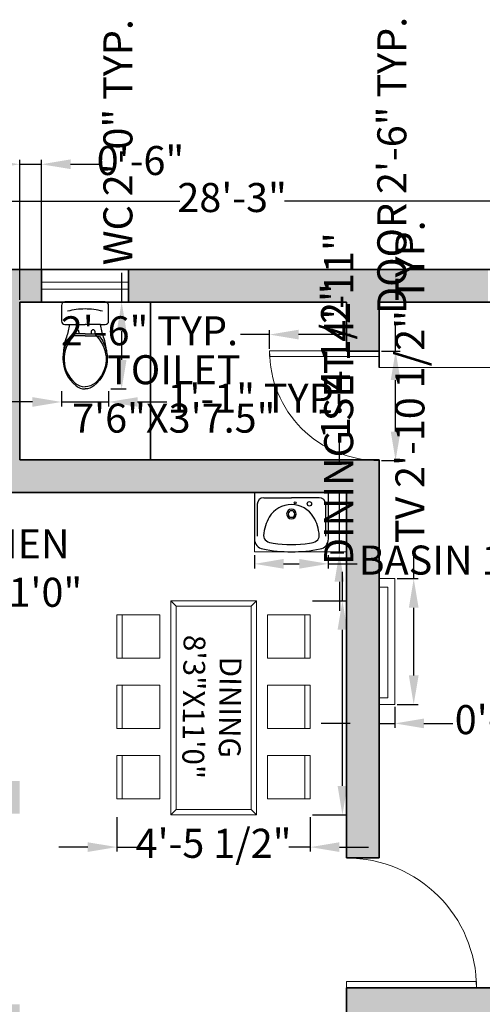
# Model space of a CAD drawing. Units: inches. Extents: x 2408 to 5087, y 2429 to 5085.
# Tile 11 of 12: x 2595 to 2723, y 2815 to 3086. Entities that reach past the tile are written whole.
import ezdxf

# ---------------------------------------------------------------- set-up
doc = ezdxf.new("R2010")
doc.units = ezdxf.units.IN
for name, color, linetype, lineweight in [('A-ANNO-DIMS', 2, 'Continuous', 18), ('A-AREA-IDEN', 6, 'Continuous', 18), ('A-DOOR', 3, 'Continuous', 18), ('A-EQPM', 53, 'Continuous', 18), ('A-FLOR-CASE', 8, 'Continuous', 18), ('A-FLOR-FIXT', 9, 'Continuous', 18), ('A-FURN', 72, 'Continuous', 18), ('A-GLAZ', 4, 'Continuous', 18), ('A-WALL', 7, 'Continuous', 35), ('A-WALL-PATT', 252, 'Continuous', 13)]:
    doc.layers.add(name, color=color, linetype=linetype, lineweight=lineweight)
for name, color, linetype in [('Washbasin-detail', 251, 'Continuous'), ('Washbasin-outline', 250, 'Continuous'), ('WC-Detail_dwgmodels.com', 251, 'Continuous'), ('WC-Outline_dwgmodels.com', 250, 'Continuous')]:
    doc.layers.add(name, color=color, linetype=linetype)
doc.styles.get("Standard").update_dxf_attribs({"font": 'arial.ttf'})
doc.dimstyles.new('ISO-25', dxfattribs={"dimtxt": 8, "dimasz": 8, "dimexe": 1.25, "dimexo": 0.625, "dimtad": 0, "dimdec": 1, "dimlunit": 4, "dimtxsty": 'Standard', "dimcen": 2.5, "dimadec": 0, "dimazin": 0, "dimtfac": 1, "dimtdec": 1, "dimtmove": 0, "dimatfit": 3, "dimfxl": 1, "dimarcsym": 0})

# ---------------------------------------------------------------- blocks, each defined once
blk = doc.blocks.new('*D1')
at = {"layer": 'A-ANNO-DIMS', "color": 0, "lineweight": -2, "transparency": 16777216}
for p, q in [((2484.49, 3017.68), (2484.49, 3037.05)), ((2492.49, 3035.8), (2639.56, 3035.8)), ((2815.49, 3035.8), (2668.43, 3035.8)), ((2823.49, 3017.68), (2823.49, 3037.05))]:
    blk.add_line(p, q, dxfattribs=at)
at = {"layer": 'A-ANNO-DIMS', "color": 0, "transparency": 16777216}
for points in [[(2492.49, 3037.13), (2492.49, 3034.47), (2484.49, 3035.8)], [(2815.49, 3037.13), (2815.49, 3034.47), (2823.49, 3035.8)]]:
    blk.add_solid(points, dxfattribs=at)
at = {"layer": 'Defpoints', "color": 0, "transparency": 16777216}
for p in [(2823.49, 3035.8), (2484.49, 3017.05), (2823.49, 3017.05)]:
    blk.add_point(p, dxfattribs=at)
at = {"layer": 'A-ANNO-DIMS', "color": 0, "transparency": 16777216, "insert": (2653.99, 3035.8), "char_height": 8, "attachment_point": 5}
blk.add_mtext('28\'-3"', dxfattribs=at)
blk = doc.blocks.new('dt')
for p, q in [((2249.04, 2869.72), (2247.08, 2871.69)), ((2278.57, 2871.69), (2276.6, 2869.72)), ((2229.22, 2850.55), (2229.22, 2866.48)), ((2296.41, 2850.55), (2296.41, 2866.48)), ((2229.22, 2824.7), (2229.22, 2840.63)), ((2296.41, 2824.7), (2296.41, 2840.63)), ((2229.22, 2798.92), (2229.22, 2814.85)), ((2296.41, 2798.92), (2296.41, 2814.85)), ((2247.08, 2792.95), (2249.04, 2794.91)), ((2278.57, 2792.95), (2276.6, 2794.91))]:
    blk.add_line(p, q)
for points in [[(2247.08, 2871.69), (2278.57, 2871.69), (2278.57, 2792.95), (2247.08, 2792.95)], [(2249.04, 2869.72), (2276.6, 2869.72), (2276.6, 2794.91), (2249.04, 2794.91)], [(2243.01, 2866.48), (2227.25, 2866.48), (2227.25, 2850.55), (2243.01, 2850.55)], [(2282.62, 2866.48), (2298.38, 2866.48), (2298.38, 2850.55), (2282.62, 2850.55)], [(2243.01, 2840.63), (2227.25, 2840.63), (2227.25, 2824.7), (2243.01, 2824.7)], [(2282.62, 2840.63), (2298.38, 2840.63), (2298.38, 2824.7), (2282.62, 2824.7)], [(2243.01, 2814.85), (2227.25, 2814.85), (2227.25, 2798.92), (2243.01, 2798.92)], [(2282.62, 2814.85), (2298.38, 2814.85), (2298.38, 2798.92), (2282.62, 2798.92)]]:
    blk.add_lwpolyline(points, close=True)
blk = doc.blocks.new('door')
blk.add_lwpolyline([(2353.25, 2862.23), (2353.25, 2898.06), (2351.47, 2898.06), (2351.47, 2862.23), (2353.25, 2862.23)])
blk.add_arc((2353.25, 2862.23), 35.83, 90, 180)
blk = doc.blocks.new('pan')
at = {"layer": 'WC-Detail_dwgmodels.com'}
for p, q in [((2600.31, 3095.45), (2600.67, 3096.11)), ((2600.67, 3096.11), (2600.67, 3096.83)), ((2601.96, 3096.11), (2600.67, 3096.11)), ((2601.96, 3096.83), (2601.96, 3096.11)), ((2604.03, 3096.11), (2601.96, 3096.11)), ((2604.03, 3096.11), (2606.1, 3096.11)), ((2606.1, 3096.83), (2606.1, 3096.11)), ((2606.1, 3096.11), (2607.39, 3096.11)), ((2607.39, 3096.11), (2607.39, 3096.83)), ((2607.75, 3095.45), (2607.39, 3096.11))]:
    blk.add_line(p, q, dxfattribs=at)
for points in [[(2600.31, 3095.45, 0.008985), (2600.04, 3095.18, 0.182634)], [(2604.03, 3095.45), (2600.31, 3095.45, 0.008985)], [(2604.03, 3095.45), (2607.75, 3095.45, -0.444938)], [(2607.75, 3095.45, -0.008985), (2608.02, 3095.18, -0.182634)], [(2600.04, 3095.18, 0.434217), (2600.67, 3079.55, 0.182634), (2604.03, 3078.32, 2.693815)], [(2599.14, 3095.18, 0.094048), (2597.09, 3091.32, 0.16845)], [(2600.04, 3095.18), (2599.14, 3095.18, 0.416606)], [(2608.02, 3095.18, -0.434217), (2607.39, 3079.55, -0.182634), (2604.03, 3078.32, -2.693815)], [(2608.02, 3095.18), (2608.92, 3095.18, -0.416606)], [(2608.92, 3095.18, -0.105447), (2611.12, 3090.81, -0.16845)], [(2597.09, 3091.32, 0.026594), (2596.78, 3090.11, 0.16845)], [(2611.12, 3090.81, -0.015301), (2611.28, 3090.11, -0.16845)]]:
    blk.add_lwpolyline(points, format="xyb", dxfattribs=at)
for centre, radius, start, end in [((2604.04, 3081.23), 23.26, 90.028, 104.6712), ((2604.02, 3081.23), 23.26, 75.3288, 89.972), ((2601.32, 3096.83), 0.645, 0, 180), ((2606.74, 3096.83), 0.645, 0, 180)]:
    blk.add_arc(centre, radius, start, end, dxfattribs=at)
at = {"layer": 'WC-Outline_dwgmodels.com'}
for points in [[(2610.82, 3099.25, 0.414214), (2611.96, 3100.39), (2611.96, 3105.7, 0.414214), (2610.82, 3106.84), (2604.03, 3106.84), (2597.24, 3106.84, 0.414214), (2596.1, 3105.7), (2596.1, 3100.39, 0.414214), (2597.24, 3099.25), (2598.79, 3099.25, -0.052345), (2597.77, 3095.01, 0.071131), (2596.78, 3090.11, 0.160777)], [(2598.79, 3099.25), (2604.03, 3099.25, 0.414214)], [(2609.26, 3099.25), (2604.03, 3099.25, -0.414214)], [(2611.28, 3090.11, 0.071131), (2610.29, 3095.01, -0.052345), (2609.26, 3099.25), (2610.82, 3099.25, 0.414214)], [(2596.78, 3090.11, 0.048023), (2596.56, 3087.87, 0.16845)], [(2611.28, 3090.11, -0.048023), (2611.5, 3087.87, -0.16845)], [(2596.56, 3087.87, 0.230343), (2601.03, 3078.62, 0.16845), (2604.03, 3077.58, 2.883082)], [(2611.5, 3087.87, -0.230343), (2607.03, 3078.62, -0.16845), (2604.03, 3077.58, -2.883082)]]:
    blk.add_lwpolyline(points, format="xyb", dxfattribs=at)
blk = doc.blocks.new('wash')
at = {"layer": 'Washbasin-detail'}
for p, q in [((2688.11, 3068.69), (2695.55, 3068.69)), ((2702.99, 3068.69), (2695.55, 3068.69)), ((2686.34, 3066.92), (2686.34, 3058.34)), ((2704.76, 3066.92), (2704.76, 3058.34))]:
    blk.add_line(p, q, dxfattribs=at)
for centre, radius in [((2696.57, 3067.33), 0.263), ((2700.39, 3067.04), 0.591)]:
    blk.add_circle(centre, radius, dxfattribs=at)
for centre, radius, start, end in [((2688.11, 3066.92), 1.77, 90, 180), ((2702.99, 3066.92), 1.77, 0, 90), ((2695.55, 3064.29), 1.28, 90, 270), ((2695.55, 3064.29), 0.886, 90, 270), ((2695.55, 3064.29), 1.28, 270, 90), ((2695.55, 3064.29), 0.886, 270, 90)]:
    blk.add_arc(centre, radius, start, end, dxfattribs=at)
at = {"layer": 'Washbasin-outline'}
for p, q in [((2685.63, 3069.93), (2685.63, 3057.59)), ((2685.77, 3070.07), (2705.33, 3070.07)), ((2705.47, 3069.93), (2705.47, 3057.59))]:
    blk.add_line(p, q, dxfattribs=at)
for centre, radius, start, end in [((2685.77, 3069.93), 0.138, 90, 180), ((2705.33, 3069.93), 0.138, 0, 90), ((2695.55, 3059.91), 6.93, 30.9425, 149.0575), ((2699.06, 3057.81), 11.02, 149.0575, 176.3179), ((2692.04, 3057.81), 11.02, 3.6821, 30.9425), ((2688.38, 3057.59), 2.76, 180, 258.7144), ((2689.63, 3058.41), 1.57, 176.3179, 238.5687), ((2691.27, 3061.1), 4.72, 238.5687, 262.476), ((2699.83, 3061.1), 4.72, 277.524, 301.4313), ((2701.47, 3058.41), 1.57, 301.4313, 3.6821), ((2702.72, 3057.59), 2.76, 281.2856, 0), ((2695.55, 3093.5), 39.37, 258.7144, 281.2856), ((2695.55, 3093.5), 37.4, 262.476, 277.524)]:
    blk.add_arc(centre, radius, start, end, dxfattribs=at)
blk = doc.blocks.new('WIN-24x9')
for p, q in [((0, 5.5), (24, 5.5)), ((0, 3.5), (24, 3.5))]:
    blk.add_line(p, q)
blk.add_lwpolyline([(0, 9), (24, 9), (24, 0), (0, 0)], close=True)
blk = doc.blocks.new('TV-FLAT-PANEL')
for points in [[(0, 34.68), (4.32, 34.68), (4.32, 0), (0, 0)], [(0, 32.31), (2.36, 32.31), (2.36, 1.87), (0, 1.87)]]:
    blk.add_lwpolyline(points, close=True)
blk = doc.blocks.new('*D41')
at = {"layer": 'A-ANNO-DIMS', "color": 0, "lineweight": -2, "transparency": 16777216}
for p, q in [((2699.02, 2994.55), (2699.02, 3002.55)), ((2695.12, 2994.55), (2700.27, 2994.55)), ((2699.02, 2972.37), (2699.02, 2986.55)), ((2695.12, 2964.37), (2700.27, 2964.37))]:
    blk.add_line(p, q, dxfattribs=at)
at = {"layer": 'A-ANNO-DIMS', "color": 0, "transparency": 16777216}
for points in [[(2697.69, 2986.55), (2700.36, 2986.55), (2699.02, 2994.55)], [(2697.69, 2972.37), (2700.36, 2972.37), (2699.02, 2964.37)]]:
    blk.add_solid(points, dxfattribs=at)
at = {"layer": 'Defpoints', "color": 0, "transparency": 16777216}
for p in [(2694.49, 2994.55), (2699.02, 2994.55), (2694.49, 2964.37)]:
    blk.add_point(p, dxfattribs=at)
at = {"layer": 'A-ANNO-DIMS', "color": 0, "transparency": 16777216, "insert": (2699.02, 3045.68), "char_height": 8, "attachment_point": 5, "rotation": 90}
blk.add_mtext('DOOR 2\'-6" TYP.', dxfattribs=at)
blk = doc.blocks.new('*D42')
at = {"layer": 'A-ANNO-DIMS', "color": 0, "lineweight": -2, "transparency": 16777216}
for p, q in [((2664.3, 2999.08), (2656.3, 2999.08)), ((2664.3, 2995.18), (2664.3, 3000.33)), ((2686.49, 2999.08), (2672.3, 2999.08)), ((2694.49, 2995.18), (2694.49, 3000.33))]:
    blk.add_line(p, q, dxfattribs=at)
at = {"layer": 'A-ANNO-DIMS', "color": 0, "transparency": 16777216}
for points in [[(2672.3, 3000.42), (2672.3, 2997.75), (2664.3, 2999.08)], [(2686.49, 3000.42), (2686.49, 2997.75), (2694.49, 2999.08)]]:
    blk.add_solid(points, dxfattribs=at)
at = {"layer": 'Defpoints', "color": 0, "transparency": 16777216}
for p in [(2664.3, 2999.08), (2664.3, 2994.55), (2694.49, 2994.55)]:
    blk.add_point(p, dxfattribs=at)
at = {"layer": 'A-ANNO-DIMS', "color": 0, "transparency": 16777216, "insert": (2631.23, 2999.08), "char_height": 8, "attachment_point": 5}
blk.add_mtext('2\'-6" TYP.', dxfattribs=at)
blk = doc.blocks.new('*D47')
at = {"layer": 'A-ANNO-DIMS', "color": 0, "lineweight": -2, "transparency": 16777216}
for p, q in [((2623.58, 3008.05), (2623.58, 3016.05)), ((2620.61, 3008.05), (2624.83, 3008.05)), ((2623.58, 2992.1), (2623.58, 3000.05)), ((2620.61, 2984.1), (2624.83, 2984.1))]:
    blk.add_line(p, q, dxfattribs=at)
at = {"layer": 'A-ANNO-DIMS', "color": 0, "transparency": 16777216}
for points in [[(2622.24, 3000.05), (2624.91, 3000.05), (2623.58, 3008.05)], [(2622.24, 2992.1), (2624.91, 2992.1), (2623.58, 2984.1)]]:
    blk.add_solid(points, dxfattribs=at)
at = {"layer": 'Defpoints', "color": 0, "transparency": 16777216}
for p in [(2619.98, 3008.05), (2623.58, 3008.05), (2619.98, 2984.1)]:
    blk.add_point(p, dxfattribs=at)
at = {"layer": 'A-ANNO-DIMS', "color": 0, "transparency": 16777216, "insert": (2623.58, 3052.09), "char_height": 8, "attachment_point": 5, "rotation": 90}
blk.add_mtext('WC 2\'-0" TYP.', dxfattribs=at)
blk = doc.blocks.new('*D48')
at = {"layer": 'A-ANNO-DIMS', "color": 0, "lineweight": -2, "transparency": 16777216}
for p, q in [((2607, 2983.48), (2607, 2979.26)), ((2619.98, 2983.48), (2619.98, 2979.26)), ((2599, 2980.51), (2591, 2980.51)), ((2607, 2980.51), (2619.98, 2980.51)), ((2627.98, 2980.51), (2635.98, 2980.51))]:
    blk.add_line(p, q, dxfattribs=at)
at = {"layer": 'A-ANNO-DIMS', "color": 0, "transparency": 16777216}
for points in [[(2599, 2981.84), (2599, 2979.18), (2607, 2980.51)], [(2627.98, 2981.84), (2627.98, 2979.18), (2619.98, 2980.51)]]:
    blk.add_solid(points, dxfattribs=at)
at = {"layer": 'Defpoints', "color": 0, "transparency": 16777216}
for p in [(2607, 2984.1), (2619.98, 2984.1), (2619.98, 2980.51)]:
    blk.add_point(p, dxfattribs=at)
at = {"layer": 'A-ANNO-DIMS', "color": 0, "transparency": 16777216, "insert": (2660.61, 2980.51), "char_height": 8, "attachment_point": 5}
blk.add_mtext('1\'-1" TYP.', dxfattribs=at)
blk = doc.blocks.new('*D49')
at = {"layer": 'A-ANNO-DIMS', "color": 0, "lineweight": -2, "transparency": 16777216}
for p, q in [((2704.01, 2931.83), (2704.01, 2939.83)), ((2699.44, 2931.83), (2705.26, 2931.83)), ((2704.01, 2905.15), (2704.01, 2923.83)), ((2699.44, 2897.15), (2705.26, 2897.15))]:
    blk.add_line(p, q, dxfattribs=at)
at = {"layer": 'A-ANNO-DIMS', "color": 0, "transparency": 16777216}
for points in [[(2702.68, 2923.83), (2705.35, 2923.83), (2704.01, 2931.83)], [(2702.68, 2905.15), (2705.35, 2905.15), (2704.01, 2897.15)]]:
    blk.add_solid(points, dxfattribs=at)
at = {"layer": 'Defpoints', "color": 0, "transparency": 16777216}
for p in [(2698.81, 2931.83), (2704.01, 2931.83), (2698.81, 2897.15)]:
    blk.add_point(p, dxfattribs=at)
at = {"layer": 'A-ANNO-DIMS', "color": 0, "transparency": 16777216, "insert": (2704.01, 2986.06), "char_height": 8, "attachment_point": 5, "rotation": 90}
blk.add_mtext('TV 2\'-10 1/2" TYP.', dxfattribs=at)
blk = doc.blocks.new('*D50')
at = {"layer": 'A-ANNO-DIMS', "color": 0, "lineweight": -2, "transparency": 16777216}
for p, q in [((2694.49, 2896.53), (2694.49, 2890.7)), ((2698.81, 2896.53), (2698.81, 2890.7)), ((2686.49, 2891.95), (2678.49, 2891.95)), ((2694.49, 2891.95), (2698.81, 2891.95)), ((2706.81, 2891.95), (2714.81, 2891.95))]:
    blk.add_line(p, q, dxfattribs=at)
at = {"layer": 'A-ANNO-DIMS', "color": 0, "transparency": 16777216}
for points in [[(2686.49, 2893.28), (2686.49, 2890.62), (2694.49, 2891.95)], [(2706.81, 2893.28), (2706.81, 2890.62), (2698.81, 2891.95)]]:
    blk.add_solid(points, dxfattribs=at)
at = {"layer": 'Defpoints', "color": 0, "transparency": 16777216}
for p in [(2694.49, 2897.15), (2698.81, 2897.15), (2698.81, 2891.95)]:
    blk.add_point(p, dxfattribs=at)
at = {"layer": 'A-ANNO-DIMS', "color": 0, "transparency": 16777216, "insert": (2749.14, 2891.95), "char_height": 8, "attachment_point": 5}
blk.add_mtext('0\'-4 1/2" TYP.', dxfattribs=at)
blk = doc.blocks.new('*D51')
at = {"layer": 'A-ANNO-DIMS', "color": 0, "lineweight": -2, "transparency": 16777216}
for p, q in [((2684.38, 2925.73), (2684.38, 2933.73)), ((2676.16, 2925.73), (2685.63, 2925.73)), ((2684.38, 2874.72), (2684.38, 2917.73)), ((2676.16, 2866.72), (2685.63, 2866.72))]:
    blk.add_line(p, q, dxfattribs=at)
at = {"layer": 'A-ANNO-DIMS', "color": 0, "transparency": 16777216}
for points in [[(2683.05, 2917.73), (2685.72, 2917.73), (2684.38, 2925.73)], [(2683.05, 2874.72), (2685.72, 2874.72), (2684.38, 2866.72)]]:
    blk.add_solid(points, dxfattribs=at)
at = {"layer": 'Defpoints', "color": 0, "transparency": 16777216}
for p in [(2675.53, 2925.73), (2684.38, 2925.73), (2675.53, 2866.72)]:
    blk.add_point(p, dxfattribs=at)
at = {"layer": 'A-ANNO-DIMS', "color": 0, "transparency": 16777216, "insert": (2684.38, 2981.42), "char_height": 8, "attachment_point": 5, "rotation": 90}
blk.add_mtext('DINING SET 4\'-11"', dxfattribs=at)
blk = doc.blocks.new('*D52')
at = {"layer": 'A-ANNO-DIMS', "color": 0, "lineweight": -2, "transparency": 16777216}
for p, q in [((2622.23, 2866.1), (2622.23, 2856.62)), ((2675.53, 2866.1), (2675.53, 2856.62)), ((2614.23, 2857.87), (2606.23, 2857.87)), ((2622.23, 2857.87), (2628.14, 2857.87)), ((2675.53, 2857.87), (2669.62, 2857.87)), ((2683.53, 2857.87), (2691.53, 2857.87))]:
    blk.add_line(p, q, dxfattribs=at)
at = {"layer": 'A-ANNO-DIMS', "color": 0, "transparency": 16777216}
for points in [[(2614.23, 2859.2), (2614.23, 2856.54), (2622.23, 2857.87)], [(2683.53, 2859.2), (2683.53, 2856.54), (2675.53, 2857.87)]]:
    blk.add_solid(points, dxfattribs=at)
at = {"layer": 'Defpoints', "color": 0, "transparency": 16777216}
for p in [(2622.23, 2866.72), (2675.53, 2866.72), (2675.53, 2857.87)]:
    blk.add_point(p, dxfattribs=at)
at = {"layer": 'A-ANNO-DIMS', "color": 0, "transparency": 16777216, "insert": (2648.88, 2857.87), "char_height": 8, "attachment_point": 5}
blk.add_mtext('4\'-5 1/2"', dxfattribs=at)
blk = doc.blocks.new('*D59')
at = {"layer": 'A-ANNO-DIMS', "color": 0, "lineweight": -2, "transparency": 16777216}
for p, q in [((2660.16, 2938.34), (2660.16, 2934.66)), ((2680.48, 2938.34), (2680.48, 2934.66)), ((2668.16, 2935.91), (2672.48, 2935.91)), ((2680.48, 2935.91), (2688.48, 2935.91))]:
    blk.add_line(p, q, dxfattribs=at)
at = {"layer": 'A-ANNO-DIMS', "color": 0, "transparency": 16777216}
for points in [[(2668.16, 2937.25), (2668.16, 2934.58), (2660.16, 2935.91)], [(2672.48, 2937.25), (2672.48, 2934.58), (2680.48, 2935.91)]]:
    blk.add_solid(points, dxfattribs=at)
at = {"layer": 'Defpoints', "color": 0, "transparency": 16777216}
for p in [(2660.16, 2938.96), (2680.48, 2938.96), (2680.48, 2935.91)]:
    blk.add_point(p, dxfattribs=at)
at = {"layer": 'A-ANNO-DIMS', "color": 0, "transparency": 16777216, "insert": (2727.21, 2935.91), "char_height": 8, "attachment_point": 5}
blk.add_mtext('BASIN 1\'-8 1/2"', dxfattribs=at)
blk = doc.blocks.new('*D60')
at = {"layer": 'A-ANNO-DIMS', "color": 0, "lineweight": -2, "transparency": 16777216}
for p, q in [((2683.53, 2963.55), (2683.53, 2971.55)), ((2681.11, 2955.55), (2684.78, 2955.55)), ((2683.53, 2938.96), (2683.53, 2955.55)), ((2681.11, 2938.96), (2684.78, 2938.96)), ((2683.53, 2930.96), (2683.53, 2922.96))]:
    blk.add_line(p, q, dxfattribs=at)
at = {"layer": 'A-ANNO-DIMS', "color": 0, "transparency": 16777216}
for points in [[(2682.2, 2963.55), (2684.87, 2963.55), (2683.53, 2955.55)], [(2682.2, 2930.96), (2684.87, 2930.96), (2683.53, 2938.96)]]:
    blk.add_solid(points, dxfattribs=at)
at = {"layer": 'Defpoints', "color": 0, "transparency": 16777216}
for p in [(2680.48, 2955.55), (2683.53, 2955.55), (2680.48, 2938.96)]:
    blk.add_point(p, dxfattribs=at)
at = {"layer": 'A-ANNO-DIMS', "color": 0, "transparency": 16777216, "insert": (2683.53, 2991.76), "char_height": 8, "attachment_point": 5, "rotation": 90}
blk.add_mtext('1\'-4 1/2"', dxfattribs=at)
blk = doc.blocks.new('*D70')
at = {"layer": 'A-ANNO-DIMS', "color": 0, "lineweight": -2, "transparency": 16777216}
for p, q in [((2595.49, 3008.68), (2595.49, 3047.25)), ((2601.49, 3008.68), (2601.49, 3047.25)), ((2587.49, 3046), (2579.49, 3046)), ((2595.49, 3046), (2601.49, 3046)), ((2609.49, 3046), (2617.49, 3046))]:
    blk.add_line(p, q, dxfattribs=at)
at = {"layer": 'A-ANNO-DIMS', "color": 0, "transparency": 16777216}
for points in [[(2587.49, 3047.34), (2587.49, 3044.67), (2595.49, 3046)], [(2609.49, 3047.34), (2609.49, 3044.67), (2601.49, 3046)]]:
    blk.add_solid(points, dxfattribs=at)
at = {"layer": 'Defpoints', "color": 0, "transparency": 16777216}
for p in [(2601.49, 3046), (2595.49, 3008.05), (2601.49, 3008.05)]:
    blk.add_point(p, dxfattribs=at)
at = {"layer": 'A-ANNO-DIMS', "color": 0, "transparency": 16777216, "insert": (2628.75, 3046), "char_height": 8, "attachment_point": 5}
blk.add_mtext('0\'-6"', dxfattribs=at)
blk = doc.blocks.new('*D79')
at = {"layer": 'A-ANNO-DIMS', "color": 0, "lineweight": -2, "transparency": 16777216}
for p, q in [((2432.93, 2818.05), (2432.93, 2826.05)), ((2693.87, 2810.05), (2431.68, 2810.05)), ((2432.93, 2810.05), (2432.93, 2809.38)), ((2432.93, 2786.05), (2432.93, 2786.73)), ((2693.87, 2786.05), (2431.68, 2786.05)), ((2432.93, 2778.05), (2432.93, 2770.05))]:
    blk.add_line(p, q, dxfattribs=at)
at = {"layer": 'A-ANNO-DIMS', "color": 0, "transparency": 16777216}
for points in [[(2431.59, 2818.05), (2434.26, 2818.05), (2432.93, 2810.05)], [(2431.59, 2778.05), (2434.26, 2778.05), (2432.93, 2786.05)]]:
    blk.add_solid(points, dxfattribs=at)
at = {"layer": 'Defpoints', "color": 0, "transparency": 16777216}
for p in [(2432.93, 2810.05), (2694.49, 2810.05), (2694.49, 2786.05)]:
    blk.add_point(p, dxfattribs=at)
at = {"layer": 'A-ANNO-DIMS', "color": 0, "transparency": 16777216, "insert": (2432.93, 2798.05), "char_height": 8, "attachment_point": 5, "rotation": 90}
blk.add_mtext('2\'-0"', dxfattribs=at)

msp = doc.modelspace()

# ---------------------------------------------------------------- hatches: boundary and pattern name
at = {"layer": 'A-WALL-PATT'}
h = msp.add_hatch(color=256, dxfattribs=at)
h.dxf.hatch_style = 1
h.paths.add_polyline_path([(2493.49, 2613.55), (2523.49, 2613.55), (2523.49, 2622.55), (2493.49, 2622.55), (2493.49, 2714.8), (2484.49, 2714.8), (2484.49, 2497.75), (2493.49, 2497.75)])
h.paths.add_polyline_path([(2613.49, 2615.42), (2613.49, 2622.55), (2583.49, 2622.55), (2583.49, 2613.55), (2613.46, 2613.55, -0.009707)])
h.paths.add_polyline_path([(2823.49, 2634.55), (2814.49, 2634.55), (2814.49, 2622.55), (2694.49, 2622.55), (2694.49, 2670.55), (2706.49, 2670.55), (2706.49, 2675.05), (2694.49, 2675.05), (2694.49, 2750.05), (2685.49, 2750.05), (2685.49, 2622.55), (2661.49, 2622.55), (2661.49, 2613.55), (2814.49, 2613.55), (2814.49, 2522.05), (2688.49, 2522.05), (2688.49, 2513.05), (2823.49, 2513.05)])
h.paths.add_polyline_path([(2823.49, 2837.05), (2814.49, 2837.05), (2814.49, 2819.05), (2685.49, 2819.05), (2685.49, 2786.05), (2694.49, 2786.05), (2694.49, 2810.05), (2814.49, 2810.05), (2814.49, 2772.55), (2823.49, 2772.55)])
h.paths.add_polyline_path([(2694.49, 2964.55), (2595.49, 2964.55), (2595.49, 3008.05), (2601.49, 3008.05), (2601.49, 3017.05), (2484.49, 3017.05), (2484.49, 2972.05), (2493.49, 2972.05), (2493.49, 3008.05), (2586.49, 3008.05), (2586.49, 2955.55), (2685.49, 2955.55), (2685.49, 2854.87), (2694.49, 2854.87)])
h.paths.add_polyline_path([(2493.49, 2867.05), (2595.49, 2867.05), (2595.49, 2876.05), (2493.49, 2876.05), (2493.49, 2912.05), (2484.49, 2912.05), (2484.49, 2774.8), (2493.49, 2774.8)])
h.paths.add_polyline_path([(2595.49, 2814.55), (2493.49, 2814.55), (2493.49, 2810.05), (2595.49, 2810.05)], flags=17)
h.paths.add_polyline_path([(2724.49, 3017.05), (2625.49, 3017.05), (2625.49, 3008.05), (2685.49, 3008.05), (2685.49, 2994.55), (2694.49, 2994.55), (2694.49, 3008.05), (2724.49, 3008.05)])
h.paths.add_polyline_path([(2823.49, 3017.05), (2784.49, 3017.05), (2784.49, 3008.05), (2814.49, 3008.05), (2814.49, 2913.55), (2814.56, 2897.05), (2823.49, 2897.05)])
h.paths.add_polyline_path([(2823.49, 2712.55), (2814.61, 2712.55), (2814.66, 2701.27), (2814.49, 2701.27), (2814.49, 2675.05), (2740.99, 2675.05), (2740.99, 2687.05), (2736.49, 2687.05), (2736.49, 2670.55), (2814.49, 2670.55), (2814.49, 2658.55), (2823.49, 2658.55)], flags=17)

# ---------------------------------------------------------------- linework, layer by layer
at = {"layer": 'A-FLOR-CASE'}
for p, q in [((2814.49, 2990.05), (2694.49, 2990.05)), ((2660.16, 2939.22), (2660.16, 2955.55)), ((2685.49, 2939.22), (2660.16, 2939.22)), ((2670.32, 2939.22), (2685.49, 2939.22))]:
    msp.add_line(p, q, dxfattribs=at)
at = {"layer": 'A-WALL'}
for p, q in [((2823.49, 3017.05), (2484.49, 3017.05)), ((2601.49, 3008.05), (2601.49, 3017.05)), ((2625.49, 3008.05), (2625.49, 3017.05)), ((2595.49, 3008.05), (2595.49, 2964.55)), ((2685.49, 3008.05), (2595.49, 3008.05)), ((2631.49, 3008.05), (2631.49, 2964.55)), ((2685.49, 3008.05), (2685.49, 2994.55)), ((2814.49, 3008.05), (2694.49, 3008.05)), ((2694.49, 3008.05), (2694.49, 2990.05)), ((2694.49, 2994.55), (2685.49, 2994.55)), ((2694.49, 2964.55), (2595.49, 2964.55)), ((2694.49, 2964.55), (2694.49, 2854.87)), ((2685.49, 2955.55), (2586.49, 2955.55)), ((2685.49, 2955.55), (2685.49, 2854.87)), ((2685.49, 2854.87), (2694.49, 2854.87)), ((2814.49, 2819.05), (2685.49, 2819.05)), ((2685.49, 2819.05), (2685.49, 2786.05))]:
    msp.add_line(p, q, dxfattribs=at)

# ---------------------------------------------------------------- block references
at = {"layer": 'A-DOOR'}
for p, xscale, yscale, zscale, rotation in [((5106.34, 1011.61), 0.8426439767912587, 0.8426439767912587, 0.8426439767912587, 89.99999999999999), ((-175.85, 5171.56), 0.9996876399039416, 0.9996876399039416, 0.9996876399039416, 270)]:
    msp.add_blockref('door', p, dxfattribs=dict(at, xscale=xscale, yscale=yscale, zscale=zscale, rotation=rotation))
at = {"layer": 'A-EQPM'}
msp.add_blockref('TV-FLAT-PANEL', (2694.49, 2897.15), dxfattribs=at)
at = {"layer": 'A-FLOR-FIXT'}
for name, p, xscale, yscale, zscale in [('pan', (481.89, 464.87), 0.8185776537930713, 0.8185776537930713, 0.8185776537930713), ('wash', (-90.58, -188.95), 1.024246129538866, 1.024246129538866, 1.024246129538866)]:
    msp.add_blockref(name, p, dxfattribs=dict(at, xscale=xscale, yscale=yscale, zscale=zscale))
at = {"layer": 'A-FURN', "xscale": 0.7493605102174018, "yscale": 0.7493605102174018, "zscale": 0.7493605102174018}
msp.add_blockref('dt', (953.22, 773.8), dxfattribs=at)
at = {"layer": 'A-GLAZ'}
msp.add_blockref('WIN-24x9', (2601.49, 3008.05), dxfattribs=at)

# ---------------------------------------------------------------- texts
at = {"layer": 'A-AREA-IDEN', "char_height": 8, "attachment_point": 1}
for s, insert in [('\\pxqc;TOILET\\P7\'6"X3\'7.5"', (2586.49, 2993.4)), ('\\pxqc;KITCHEN\\P7\'9"X11\'0"', (2534.8, 2945.41))]:
    msp.add_mtext_dynamic_manual_height_columns(s, width=102.8772, gutter_width=12.5, heights=[0], dxfattribs=dict(at, insert=insert))
at = {"layer": 'A-AREA-IDEN', "insert": (2656.98, 2947.79), "char_height": 6, "attachment_point": 1, "rotation": 269.4083}
msp.add_mtext_dynamic_manual_height_columns('\\pxqc;DINING\\P8\'3"X11\'0"', width=102.8772, gutter_width=12.5, heights=[0], dxfattribs=at)

# ---------------------------------------------------------------- dimensions: what is measured, and where the dimension line sits
at = {"layer": 'A-ANNO-DIMS'}
for base, p1, p2, angle, text, picture, middle in [((2623.5769, 3008.0542), (2619.9841, 2984.1021), (2619.9841, 3008.0542), 90, 'WC <> TYP.', '*D47', (2623.5769, 3052.0871)), ((2699.02, 2994.55), (2694.49, 2964.37), (2694.49, 2994.55), 90, 'DOOR <> TYP.', '*D41', (2699.02, 3045.68)), ((2704.01, 2931.83), (2698.81, 2897.15), (2698.81, 2931.83), 90, 'TV <> TYP.', '*D49', (2704.01, 2986.06)), ((2684.38, 2925.73), (2675.53, 2866.72), (2675.53, 2925.73), 90, 'DINING SET <>', '*D51', (2684.38, 2981.42)), ((2664.3, 2999.08), (2694.49, 2994.55), (2664.3, 2994.55), 180, '<> TYP.', '*D42', (2631.23, 2999.08))]:
    dim = msp.add_linear_dim(base=base, p1=p1, p2=p2, angle=angle, text=text, dimstyle='ISO-25', override={"dimdec": 1, "dimlfac": 1, "dimrnd": 0, "dimzin": 1, "dimdsep": 46, "dimlunit": 4, "dimfrac": 2}, dxfattribs=at)
    dim.commit()
    dim.dimension.update_dxf_attribs({"geometry": picture, "text_midpoint": middle})
for base, p1, p2, override, picture, middle in [((2601.49, 3046), (2595.49, 3008.05), (2601.49, 3008.05), {"dimdec": 1, "dimlfac": 1, "dimrnd": 0, "dimzin": 1, "dimdsep": 46, "dimlunit": 4, "dimfrac": 2}, '*D70', (2628.75, 3046)), ((2823.49, 3035.8), (2484.49, 3017.05), (2823.49, 3017.05), {"dimclrd": 0, "dimclre": 0, "dimclrt": 0}, '*D1', (2653.99, 3035.8)), ((2675.53, 2857.87), (2622.23, 2866.72), (2675.53, 2866.72), {"dimdec": 1, "dimlfac": 1, "dimrnd": 0, "dimzin": 1, "dimdsep": 46, "dimlunit": 4, "dimfrac": 2}, '*D52', (2648.88, 2857.87))]:
    dim = msp.add_linear_dim(base=base, p1=p1, p2=p2, dimstyle='ISO-25', override=override, dxfattribs=at)
    dim.commit()
    dim.dimension.update_dxf_attribs({"geometry": picture, "text_midpoint": middle})
for base, p1, p2, picture, middle in [((2683.53, 2955.55), (2680.48, 2938.96), (2680.48, 2955.55), '*D60', (2683.53, 2991.76)), ((2432.93, 2810.05), (2694.49, 2786.05), (2694.49, 2810.05), '*D79', (2432.93, 2798.05))]:
    dim = msp.add_linear_dim(base=base, p1=p1, p2=p2, angle=90, dimstyle='ISO-25', override={"dimdec": 1, "dimlfac": 1, "dimrnd": 0, "dimzin": 1, "dimdsep": 46, "dimlunit": 4, "dimfrac": 2}, dxfattribs=at)
    dim.commit()
    dim.dimension.update_dxf_attribs({"geometry": picture, "text_midpoint": middle})
for base, p1, p2, text, picture, middle in [((2619.98, 2980.51), (2607, 2984.1), (2619.98, 2984.1), '<> TYP.', '*D48', (2660.61, 2980.51)), ((2680.48, 2935.91), (2660.16, 2938.96), (2680.48, 2938.96), 'BASIN <>', '*D59', (2727.21, 2935.91)), ((2698.81, 2891.95), (2694.49, 2897.15), (2698.81, 2897.15), '<> TYP.', '*D50', (2749.14, 2891.95))]:
    dim = msp.add_linear_dim(base=base, p1=p1, p2=p2, text=text, dimstyle='ISO-25', override={"dimdec": 1, "dimlfac": 1, "dimrnd": 0, "dimzin": 1, "dimdsep": 46, "dimlunit": 4, "dimfrac": 2}, dxfattribs=at)
    dim.commit()
    dim.dimension.update_dxf_attribs({"geometry": picture, "text_midpoint": middle})

doc.saveas('drawing.dxf')
